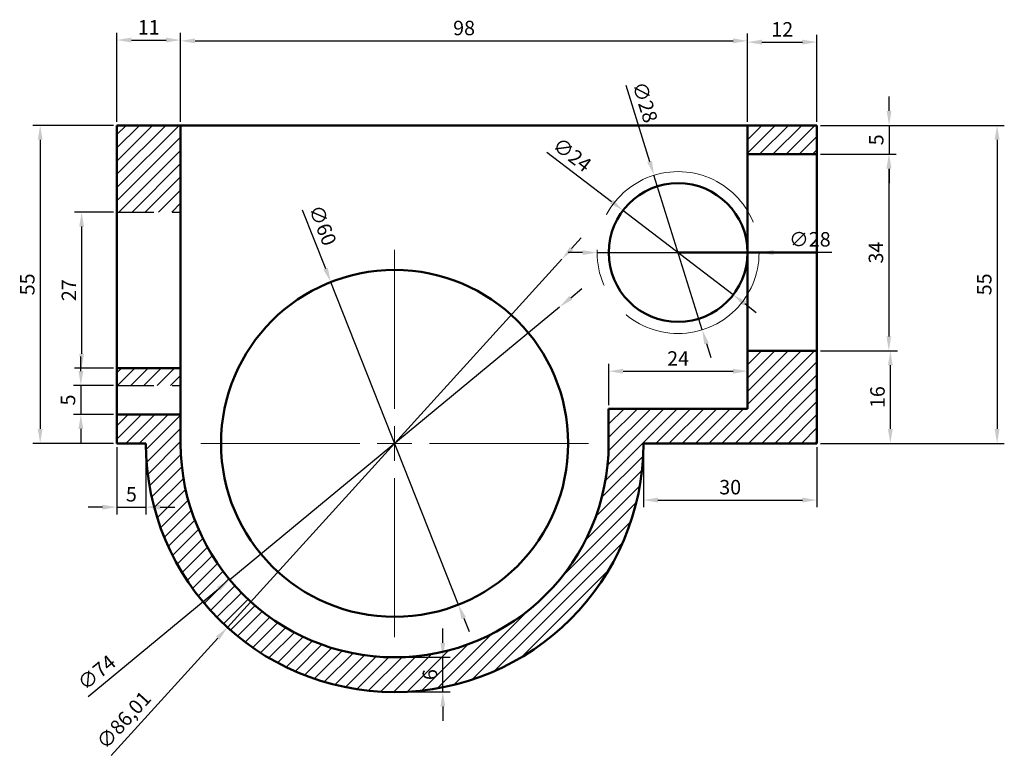
# Model space of a CAD drawing. Units: millimetres. Extents: x 1194 to 1920, y 1729 to 2086.
# Tile 5 of 5: x 1750 to 1920, y 1959 to 2086. Entities that reach past the tile are written whole.
import ezdxf

# ---------------------------------------------------------------- set-up
doc = ezdxf.new("R2010")
doc.units = ezdxf.units.MM
doc.linetypes.add('CENTER', pattern=[50.8, 31.75, -6.35, 6.35, -6.35])
doc.linetypes.add('HIDDEN', pattern=[9.525, 6.35, -3.175])
for name, color, linetype, lineweight in [('M-CNTR', 1, 'CENTER', 18), ('M-DIMS', 2, 'Continuous', 25), ('M-HATC', 8, 'Continuous', 18), ('M-HIDN', 4, 'HIDDEN', 25), ('M-OUTL', 7, 'Continuous', 50)]:
    doc.layers.add(name, color=color, linetype=linetype, lineweight=lineweight)
doc.styles.get("Standard").update_dxf_attribs({"font": 'arial.ttf'})
doc.dimstyles.new('ISO-25', dxfattribs={"dimtxt": 2.5, "dimasz": 2.5, "dimexe": 1.25, "dimexo": 0.625, "dimtad": 1, "dimtxsty": 'Standard', "dimcen": 2.5, "dimadec": 0, "dimazin": 0, "dimtfac": 1, "dimtmove": 0, "dimatfit": 3, "dimfxl": 1, "dimarcsym": 0})

# ---------------------------------------------------------------- blocks, each defined once
blk = doc.blocks.new('*U9')
at = {"layer": 'M-CNTR', "color": 0, "transparency": 16777216}
for p, q in [((0, 6), (0, 33.5)), ((-33.5, 0), (-6, 0)), ((6, 0), (33.5, 0)), ((0, -33.5), (0, -6))]:
    blk.add_line(p, q, dxfattribs=at)
at = {"layer": 'M-CNTR', "color": 0, "linetype": 'Continuous', "transparency": 16777216}
for p, q in [((0, -3), (0, 3)), ((-3, 0), (3, 0))]:
    blk.add_line(p, q, dxfattribs=at)
blk = doc.blocks.new('*D62')
at = {"layer": 'Defpoints', "color": 0, "transparency": 16777216}
for p in [(1777.47, 2082.79), (1766.46, 2068.03), (1777.47, 2068.03)]:
    blk.add_point(p, dxfattribs=at)
at = {"layer": 'M-DIMS', "color": 0, "lineweight": -2, "transparency": 16777216}
for p, q in [((1766.46, 2068.65), (1766.46, 2084.04)), ((1777.47, 2068.65), (1777.47, 2084.04)), ((1768.96, 2082.79), (1774.97, 2082.79))]:
    blk.add_line(p, q, dxfattribs=at)
at = {"layer": 'M-DIMS', "color": 0, "transparency": 16777216}
for points in [[(1768.96, 2083.21), (1768.96, 2082.37), (1766.46, 2082.79)], [(1774.97, 2083.21), (1774.97, 2082.37), (1777.47, 2082.79)]]:
    blk.add_solid(points, dxfattribs=at)
at = {"layer": 'M-DIMS', "color": 0, "transparency": 16777216, "insert": (1771.96, 2084.67), "char_height": 2.5, "attachment_point": 5}
blk.add_mtext('11', dxfattribs=at)
blk = doc.blocks.new('*D63')
at = {"layer": 'Defpoints', "color": 0, "transparency": 16777216}
for p in [(1875.47, 2082.65), (1777.47, 2068.03), (1875.47, 2068.03)]:
    blk.add_point(p, dxfattribs=at)
at = {"layer": 'M-DIMS', "color": 0, "lineweight": -2, "transparency": 16777216}
for p, q in [((1777.47, 2068.65), (1777.47, 2083.9)), ((1875.47, 2068.65), (1875.47, 2083.9)), ((1779.97, 2082.65), (1872.97, 2082.65))]:
    blk.add_line(p, q, dxfattribs=at)
at = {"layer": 'M-DIMS', "color": 0, "transparency": 16777216}
for points in [[(1779.97, 2083.07), (1779.97, 2082.23), (1777.47, 2082.65)], [(1872.97, 2083.07), (1872.97, 2082.23), (1875.47, 2082.65)]]:
    blk.add_solid(points, dxfattribs=at)
at = {"layer": 'M-DIMS', "color": 0, "transparency": 16777216, "insert": (1826.47, 2084.55), "char_height": 2.5, "attachment_point": 5}
blk.add_mtext('98', dxfattribs=at)
blk = doc.blocks.new('*D64')
at = {"layer": 'Defpoints', "color": 0, "transparency": 16777216}
for p in [(1887.47, 2082.43), (1875.47, 2068.03), (1887.47, 2068.03)]:
    blk.add_point(p, dxfattribs=at)
at = {"layer": 'M-DIMS', "color": 0, "lineweight": -2, "transparency": 16777216}
for p, q in [((1875.47, 2068.65), (1875.47, 2083.68)), ((1887.47, 2068.65), (1887.47, 2083.68)), ((1877.97, 2082.43), (1884.97, 2082.43))]:
    blk.add_line(p, q, dxfattribs=at)
at = {"layer": 'M-DIMS', "color": 0, "transparency": 16777216}
for points in [[(1877.97, 2082.85), (1877.97, 2082.01), (1875.47, 2082.43)], [(1884.97, 2082.85), (1884.97, 2082.01), (1887.47, 2082.43)]]:
    blk.add_solid(points, dxfattribs=at)
at = {"layer": 'M-DIMS', "color": 0, "transparency": 16777216, "insert": (1881.47, 2084.31), "char_height": 2.5, "attachment_point": 5}
blk.add_mtext('12', dxfattribs=at)
blk = doc.blocks.new('*D65')
at = {"layer": 'Defpoints', "color": 0, "transparency": 16777216}
for p in [(1887.47, 2068.03), (1887.47, 2013.03), (1918.61, 2013.03)]:
    blk.add_point(p, dxfattribs=at)
at = {"layer": 'M-DIMS', "color": 0, "lineweight": -2, "transparency": 16777216}
for p, q in [((1888.09, 2068.03), (1919.86, 2068.03)), ((1918.61, 2065.53), (1918.61, 2015.53)), ((1888.09, 2013.03), (1919.86, 2013.03))]:
    blk.add_line(p, q, dxfattribs=at)
at = {"layer": 'M-DIMS', "color": 0, "transparency": 16777216}
for points in [[(1918.19, 2065.53), (1919.03, 2065.53), (1918.61, 2068.03)], [(1918.19, 2015.53), (1919.03, 2015.53), (1918.61, 2013.03)]]:
    blk.add_solid(points, dxfattribs=at)
at = {"layer": 'M-DIMS', "color": 0, "transparency": 16777216, "insert": (1916.71, 2040.53), "char_height": 2.5, "attachment_point": 5, "rotation": 90}
blk.add_mtext('55', dxfattribs=at)
blk = doc.blocks.new('*D66')
at = {"layer": 'Defpoints', "color": 0, "transparency": 16777216}
for p in [(1887.47, 2068.03), (1887.47, 2063.03), (1899.94, 2063.03)]:
    blk.add_point(p, dxfattribs=at)
at = {"layer": 'M-DIMS', "color": 0, "lineweight": -2, "transparency": 16777216}
for p, q in [((1899.94, 2070.53), (1899.94, 2073.03)), ((1888.09, 2068.03), (1901.19, 2068.03)), ((1899.94, 2068.03), (1899.94, 2063.03)), ((1888.09, 2063.03), (1901.19, 2063.03)), ((1899.94, 2060.53), (1899.94, 2058.03))]:
    blk.add_line(p, q, dxfattribs=at)
at = {"layer": 'M-DIMS', "color": 0, "transparency": 16777216}
for points in [[(1899.52, 2070.53), (1900.36, 2070.53), (1899.94, 2068.03)], [(1899.52, 2060.53), (1900.36, 2060.53), (1899.94, 2063.03)]]:
    blk.add_solid(points, dxfattribs=at)
at = {"layer": 'M-DIMS', "color": 0, "transparency": 16777216, "insert": (1898.04, 2065.53), "char_height": 2.5, "attachment_point": 5, "rotation": 90}
blk.add_mtext('5', dxfattribs=at)
blk = doc.blocks.new('*D67')
at = {"layer": 'Defpoints', "color": 0, "transparency": 16777216}
for p in [(1887.47, 2029.03), (1900.16, 2029.03), (1887.47, 2013.03)]:
    blk.add_point(p, dxfattribs=at)
at = {"layer": 'M-DIMS', "color": 0, "lineweight": -2, "transparency": 16777216}
for p, q in [((1888.09, 2029.03), (1901.41, 2029.03)), ((1900.16, 2015.53), (1900.16, 2026.53)), ((1888.09, 2013.03), (1901.41, 2013.03))]:
    blk.add_line(p, q, dxfattribs=at)
at = {"layer": 'M-DIMS', "color": 0, "transparency": 16777216}
for points in [[(1899.74, 2026.53), (1900.57, 2026.53), (1900.16, 2029.03)], [(1899.74, 2015.53), (1900.57, 2015.53), (1900.16, 2013.03)]]:
    blk.add_solid(points, dxfattribs=at)
at = {"layer": 'M-DIMS', "color": 0, "transparency": 16777216, "insert": (1898.26, 2021.03), "char_height": 2.5, "attachment_point": 5, "rotation": 90}
blk.add_mtext('16', dxfattribs=at)
blk = doc.blocks.new('*D68')
at = {"layer": 'Defpoints', "color": 0, "transparency": 16777216}
for p in [(1766.46, 2013.03), (1771.46, 2013.03), (1771.46, 2002)]:
    blk.add_point(p, dxfattribs=at)
at = {"layer": 'M-DIMS', "color": 0, "lineweight": -2, "transparency": 16777216}
for p, q in [((1766.46, 2012.4), (1766.46, 2000.75)), ((1771.46, 2012.4), (1771.46, 2000.75)), ((1763.96, 2002), (1761.46, 2002)), ((1766.46, 2002), (1771.46, 2002)), ((1773.96, 2002), (1776.46, 2002))]:
    blk.add_line(p, q, dxfattribs=at)
at = {"layer": 'M-DIMS', "color": 0, "transparency": 16777216}
for points in [[(1763.96, 2002.42), (1763.96, 2001.58), (1766.46, 2002)], [(1773.96, 2002.42), (1773.96, 2001.58), (1771.46, 2002)]]:
    blk.add_solid(points, dxfattribs=at)
at = {"layer": 'M-DIMS', "color": 0, "transparency": 16777216, "insert": (1768.96, 2003.9), "char_height": 2.5, "attachment_point": 5}
blk.add_mtext('5', dxfattribs=at)
blk = doc.blocks.new('*D69')
at = {"layer": 'Defpoints', "color": 0, "transparency": 16777216}
for p in [(1766.46, 2068.03), (1753.19, 2013.03), (1766.46, 2013.03)]:
    blk.add_point(p, dxfattribs=at)
at = {"layer": 'M-DIMS', "color": 0, "lineweight": -2, "transparency": 16777216}
for p, q in [((1765.84, 2068.03), (1751.94, 2068.03)), ((1753.19, 2065.53), (1753.19, 2015.53)), ((1765.84, 2013.03), (1751.94, 2013.03))]:
    blk.add_line(p, q, dxfattribs=at)
at = {"layer": 'M-DIMS', "color": 0, "transparency": 16777216}
for points in [[(1752.77, 2065.53), (1753.61, 2065.53), (1753.19, 2068.03)], [(1752.77, 2015.53), (1753.61, 2015.53), (1753.19, 2013.03)]]:
    blk.add_solid(points, dxfattribs=at)
at = {"layer": 'M-DIMS', "color": 0, "transparency": 16777216, "insert": (1751.29, 2040.53), "char_height": 2.5, "attachment_point": 5, "rotation": 90}
blk.add_mtext('55', dxfattribs=at)
blk = doc.blocks.new('*D70')
at = {"layer": 'Defpoints', "color": 0, "transparency": 16777216}
for p in [(1766.46, 2053.03), (1760.36, 2026.03), (1766.46, 2026.03)]:
    blk.add_point(p, dxfattribs=at)
at = {"layer": 'M-DIMS', "color": 0, "lineweight": -2, "transparency": 16777216}
for p, q in [((1765.84, 2053.03), (1759.11, 2053.03)), ((1760.36, 2050.53), (1760.36, 2028.53)), ((1765.84, 2026.03), (1759.11, 2026.03))]:
    blk.add_line(p, q, dxfattribs=at)
at = {"layer": 'M-DIMS', "color": 0, "transparency": 16777216}
for points in [[(1759.94, 2050.53), (1760.78, 2050.53), (1760.36, 2053.03)], [(1759.94, 2028.53), (1760.78, 2028.53), (1760.36, 2026.03)]]:
    blk.add_solid(points, dxfattribs=at)
at = {"layer": 'M-DIMS', "color": 0, "transparency": 16777216, "insert": (1758.48, 2039.53), "char_height": 2.5, "attachment_point": 5, "rotation": 90}
blk.add_mtext('27', dxfattribs=at)
blk = doc.blocks.new('*D71')
at = {"layer": 'Defpoints', "color": 0, "transparency": 16777216}
for p in [(1766.46, 2023.03), (1760.22, 2018.03), (1766.46, 2018.03)]:
    blk.add_point(p, dxfattribs=at)
at = {"layer": 'M-DIMS', "color": 0, "lineweight": -2, "transparency": 16777216}
for p, q in [((1760.22, 2025.53), (1760.22, 2028.03)), ((1765.84, 2023.03), (1758.97, 2023.03)), ((1760.22, 2023.03), (1760.22, 2018.03)), ((1765.84, 2018.03), (1758.97, 2018.03)), ((1760.22, 2015.53), (1760.22, 2013.03))]:
    blk.add_line(p, q, dxfattribs=at)
at = {"layer": 'M-DIMS', "color": 0, "transparency": 16777216}
for points in [[(1759.81, 2025.53), (1760.64, 2025.53), (1760.22, 2023.03)], [(1759.81, 2015.53), (1760.64, 2015.53), (1760.22, 2018.03)]]:
    blk.add_solid(points, dxfattribs=at)
at = {"layer": 'M-DIMS', "color": 0, "transparency": 16777216, "insert": (1758.33, 2020.53), "char_height": 2.5, "attachment_point": 5, "rotation": 90}
blk.add_mtext('5', dxfattribs=at)
blk = doc.blocks.new('*D72')
at = {"layer": 'Defpoints', "color": 0, "transparency": 16777216}
for p in [(1875.47, 2025.51), (1851.47, 2019.03), (1875.47, 2019.03)]:
    blk.add_point(p, dxfattribs=at)
at = {"layer": 'M-DIMS', "color": 0, "lineweight": -2, "transparency": 16777216}
for p, q in [((1851.47, 2019.65), (1851.47, 2026.76)), ((1853.97, 2025.51), (1872.97, 2025.51)), ((1875.47, 2019.65), (1875.47, 2026.76))]:
    blk.add_line(p, q, dxfattribs=at)
at = {"layer": 'M-DIMS', "color": 0, "transparency": 16777216}
for points in [[(1853.97, 2025.93), (1853.97, 2025.09), (1851.47, 2025.51)], [(1872.97, 2025.93), (1872.97, 2025.09), (1875.47, 2025.51)]]:
    blk.add_solid(points, dxfattribs=at)
at = {"layer": 'M-DIMS', "color": 0, "transparency": 16777216, "insert": (1863.47, 2027.39), "char_height": 2.5, "attachment_point": 5}
blk.add_mtext('24', dxfattribs=at)
blk = doc.blocks.new('*D73')
at = {"layer": 'Defpoints', "color": 0, "transparency": 16777216}
for p in [(1857.47, 2013.03), (1887.47, 2013.03), (1887.47, 2003.22)]:
    blk.add_point(p, dxfattribs=at)
at = {"layer": 'M-DIMS', "color": 0, "lineweight": -2, "transparency": 16777216}
for p, q in [((1857.47, 2012.4), (1857.47, 2001.97)), ((1887.47, 2012.4), (1887.47, 2001.97)), ((1859.97, 2003.22), (1884.97, 2003.22))]:
    blk.add_line(p, q, dxfattribs=at)
at = {"layer": 'M-DIMS', "color": 0, "transparency": 16777216}
for points in [[(1859.97, 2003.64), (1859.97, 2002.81), (1857.47, 2003.22)], [(1884.97, 2003.64), (1884.97, 2002.81), (1887.47, 2003.22)]]:
    blk.add_solid(points, dxfattribs=at)
at = {"layer": 'M-DIMS', "color": 0, "transparency": 16777216, "insert": (1872.47, 2005.13), "char_height": 2.5, "attachment_point": 5}
blk.add_mtext('30', dxfattribs=at)
blk = doc.blocks.new('*D74')
at = {"layer": 'Defpoints', "color": 0, "transparency": 16777216}
for p in [(1887.47, 2063.03), (1887.47, 2029.03), (1899.9, 2029.03)]:
    blk.add_point(p, dxfattribs=at)
at = {"layer": 'M-DIMS', "color": 0, "lineweight": -2, "transparency": 16777216}
for p, q in [((1888.09, 2063.03), (1901.15, 2063.03)), ((1899.9, 2060.53), (1899.9, 2031.53)), ((1888.09, 2029.03), (1901.15, 2029.03))]:
    blk.add_line(p, q, dxfattribs=at)
at = {"layer": 'M-DIMS', "color": 0, "transparency": 16777216}
for points in [[(1899.48, 2060.53), (1900.31, 2060.53), (1899.9, 2063.03)], [(1899.48, 2031.53), (1900.31, 2031.53), (1899.9, 2029.03)]]:
    blk.add_solid(points, dxfattribs=at)
at = {"layer": 'M-DIMS', "color": 0, "transparency": 16777216, "insert": (1897.99, 2046.03), "char_height": 2.5, "attachment_point": 5, "rotation": 90}
blk.add_mtext('34', dxfattribs=at)
blk = doc.blocks.new('*D75')
at = {"layer": 'Defpoints', "color": 0, "transparency": 16777216}
for p in [(1853.94, 2053.33), (1872.99, 2038.73)]:
    blk.add_point(p, dxfattribs=at)
at = {"layer": 'M-DIMS', "color": 0, "lineweight": -2, "transparency": 16777216}
for p, q in [((1840.77, 2063.42), (1851.96, 2054.85)), ((1872.99, 2038.73), (1853.94, 2053.33)), ((1874.98, 2037.21), (1876.96, 2035.69))]:
    blk.add_line(p, q, dxfattribs=at)
at = {"layer": 'M-DIMS', "color": 0, "transparency": 16777216}
for points in [[(1852.21, 2055.18), (1851.71, 2054.52), (1853.94, 2053.33)], [(1875.23, 2037.54), (1874.72, 2036.88), (1872.99, 2038.73)]]:
    blk.add_solid(points, dxfattribs=at)
at = {"layer": 'M-DIMS', "color": 0, "transparency": 16777216, "insert": (1844.96, 2062.7), "char_height": 2.5, "attachment_point": 5, "rotation": 322.5372}
blk.add_mtext('∅24', dxfattribs=at)
blk = doc.blocks.new('*D76')
at = {"layer": 'Defpoints', "color": 0, "transparency": 16777216}
for p in [(1859.3, 2059.39), (1867.64, 2032.67)]:
    blk.add_point(p, dxfattribs=at)
at = {"layer": 'M-DIMS', "color": 0, "lineweight": -2, "transparency": 16777216}
for p, q in [((1854.43, 2074.97), (1858.55, 2061.78)), ((1867.64, 2032.67), (1859.3, 2059.39)), ((1868.39, 2030.28), (1869.13, 2027.89))]:
    blk.add_line(p, q, dxfattribs=at)
at = {"layer": 'M-DIMS', "color": 0, "transparency": 16777216}
for points in [[(1858.95, 2061.9), (1858.15, 2061.66), (1859.3, 2059.39)], [(1868.78, 2030.4), (1867.99, 2030.16), (1867.64, 2032.67)]]:
    blk.add_solid(points, dxfattribs=at)
at = {"layer": 'M-DIMS', "color": 0, "transparency": 16777216, "insert": (1857.44, 2071.95), "char_height": 2.5, "attachment_point": 5, "rotation": 287.3417}
blk.add_mtext('∅28', dxfattribs=at)
blk = doc.blocks.new('*D77')
at = {"layer": 'Defpoints', "color": 0, "transparency": 16777216}
for p in [(1803.44, 2040.93), (1825.49, 1985.13)]:
    blk.add_point(p, dxfattribs=at)
at = {"layer": 'M-DIMS', "color": 0, "lineweight": -2, "transparency": 16777216}
for p, q in [((1798.51, 2053.42), (1802.52, 2043.26)), ((1825.49, 1985.13), (1803.44, 2040.93)), ((1826.41, 1982.8), (1827.33, 1980.48))]:
    blk.add_line(p, q, dxfattribs=at)
at = {"layer": 'M-DIMS', "color": 0, "transparency": 16777216}
for points in [[(1802.91, 2043.41), (1802.13, 2043.1), (1803.44, 2040.93)], [(1826.8, 1982.96), (1826.02, 1982.65), (1825.49, 1985.13)]]:
    blk.add_solid(points, dxfattribs=at)
at = {"layer": 'M-DIMS', "color": 0, "transparency": 16777216, "insert": (1801.73, 2050.63), "char_height": 2.5, "attachment_point": 5, "rotation": 291.5599}
blk.add_mtext('∅60', dxfattribs=at)
blk = doc.blocks.new('*D78')
at = {"layer": 'Defpoints', "color": 0, "transparency": 16777216}
for p in [(1842.98, 2036.61), (1785.95, 1989.45)]:
    blk.add_point(p, dxfattribs=at)
at = {"layer": 'M-DIMS', "color": 0, "lineweight": -2, "transparency": 16777216}
for p, q in [((1844.9, 2038.2), (1846.83, 2039.8)), ((1842.98, 2036.61), (1785.95, 1989.45)), ((1761.51, 1969.23), (1784.03, 1987.85))]:
    blk.add_line(p, q, dxfattribs=at)
at = {"layer": 'M-DIMS', "color": 0, "transparency": 16777216}
for points in [[(1844.64, 2038.52), (1845.17, 2037.88), (1842.98, 2036.61)], [(1783.76, 1988.18), (1784.29, 1987.53), (1785.95, 1989.45)]]:
    blk.add_solid(points, dxfattribs=at)
at = {"layer": 'M-DIMS', "color": 0, "transparency": 16777216, "insert": (1763.16, 1973.15), "char_height": 2.5, "attachment_point": 5, "rotation": 39.5929}
blk.add_mtext('∅74', dxfattribs=at)
blk = doc.blocks.new('*D79')
at = {"layer": 'Defpoints', "color": 0, "transparency": 16777216}
for p in [(1843.37, 2044.87), (1785.56, 1981.19)]:
    blk.add_point(p, dxfattribs=at)
at = {"layer": 'M-DIMS', "color": 0, "lineweight": -2, "transparency": 16777216}
for p, q in [((1845.05, 2046.72), (1846.74, 2048.57)), ((1843.37, 2044.87), (1785.56, 1981.19)), ((1765.47, 1959.07), (1783.88, 1979.34))]:
    blk.add_line(p, q, dxfattribs=at)
at = {"layer": 'M-DIMS', "color": 0, "transparency": 16777216}
for points in [[(1844.75, 2047), (1845.36, 2046.44), (1843.37, 2044.87)], [(1783.57, 1979.62), (1784.18, 1979.06), (1785.56, 1981.19)]]:
    blk.add_solid(points, dxfattribs=at)
at = {"layer": 'M-DIMS', "color": 0, "transparency": 16777216, "insert": (1767.88, 1964.95), "char_height": 2.5, "attachment_point": 5, "rotation": 47.7595}
blk.add_mtext('∅86,01', dxfattribs=at)
blk = doc.blocks.new('*D80')
at = {"layer": 'Defpoints', "color": 0, "transparency": 16777216}
for p in [(1814.47, 1976.03), (1822.79, 1976.03), (1814.47, 1970.03)]:
    blk.add_point(p, dxfattribs=at)
at = {"layer": 'M-DIMS', "color": 0, "lineweight": -2, "transparency": 16777216}
for p, q in [((1822.79, 1978.53), (1822.79, 1981.03)), ((1815.09, 1976.03), (1824.04, 1976.03)), ((1822.79, 1970.03), (1822.79, 1976.03)), ((1815.09, 1970.03), (1824.04, 1970.03)), ((1822.79, 1967.53), (1822.79, 1965.03))]:
    blk.add_line(p, q, dxfattribs=at)
at = {"layer": 'M-DIMS', "color": 0, "transparency": 16777216}
for points in [[(1822.38, 1978.53), (1823.21, 1978.53), (1822.79, 1976.03)], [(1822.38, 1967.53), (1823.21, 1967.53), (1822.79, 1970.03)]]:
    blk.add_solid(points, dxfattribs=at)
at = {"layer": 'M-DIMS', "color": 0, "transparency": 16777216, "insert": (1820.89, 1973.03), "char_height": 2.5, "attachment_point": 5, "rotation": 90}
blk.add_mtext('6', dxfattribs=at)
blk = doc.blocks.new('*D149')
at = {"layer": 'Defpoints', "color": 0, "transparency": 16777216}
for p in [(1849.47, 2046.03), (1877.47, 2046.03)]:
    blk.add_point(p, dxfattribs=at)
at = {"layer": 'M-DIMS', "color": 0, "lineweight": -2, "transparency": 16777216}
for p, q in [((1846.97, 2046.03), (1844.47, 2046.03)), ((1849.47, 2046.03), (1877.47, 2046.03)), ((1890.02, 2046.03), (1879.97, 2046.03))]:
    blk.add_line(p, q, dxfattribs=at)
at = {"layer": 'M-DIMS', "color": 0, "transparency": 16777216}
for points in [[(1846.97, 2046.45), (1846.97, 2045.61), (1849.47, 2046.03)], [(1879.97, 2046.45), (1879.97, 2045.61), (1877.47, 2046.03)]]:
    blk.add_solid(points, dxfattribs=at)
at = {"layer": 'M-DIMS', "color": 0, "transparency": 16777216, "insert": (1886.25, 2048), "char_height": 2.5, "attachment_point": 5, "rotation": 359.9988}
blk.add_mtext('∅28', dxfattribs=at)

msp = doc.modelspace()

# ---------------------------------------------------------------- hatches: boundary and pattern name
at = {"layer": 'M-HATC'}
h = msp.add_hatch(dxfattribs=at)
h.set_pattern_fill('ANSI31', color=256, scale=0.51)
h.paths.add_polyline_path([(1771.462, 2013.0293), (1766.462, 2013.0293), (1766.462, 2018.0293), (1777.4653, 2018.0293), (1777.4653, 2013.0293, 1), (1851.4653, 2013.0293), (1851.4653, 2019.0293), (1875.4685, 2019.0293), (1875.4685, 2029.0293), (1887.4685, 2029.0293), (1887.4685, 2013.0293), (1857.4685, 2013.0293, -1)])
h.paths.add_polyline_path([(1887.4685, 2068.0293), (1875.4685, 2068.0293), (1875.4685, 2063.0293), (1887.4685, 2063.0293), (1887.4685, 2066.0293)])
h = msp.add_hatch(dxfattribs=at)
h.set_pattern_fill('ANSI31', color=256, scale=0.51)
h.paths.add_polyline_path([(1777.4653, 2068.0293), (1776.462, 2068.0293), (1766.462, 2068.0293), (1766.462, 2053.0293), (1777.4653, 2053.0293)])
h.paths.add_polyline_path([(1777.4653, 2026.0293), (1766.462, 2026.0293), (1766.462, 2023.0293), (1777.4653, 2023.0293)])

# ---------------------------------------------------------------- linework, layer by layer
at = {"layer": 'M-CNTR'}
msp.add_circle((1863.4685, 2046.0293), 14, dxfattribs=at)
at = {"layer": 'M-HIDN'}
for p, q in [((1766.462, 2068.0293), (1766.462, 2053.0293)), ((1766.462, 2053.0293), (1777.4653, 2053.0293)), ((1766.462, 2018.0293), (1766.462, 2023.0293)), ((1766.462, 2023.0293), (1777.4653, 2023.0293))]:
    msp.add_line(p, q, dxfattribs=at)
at = {"layer": 'M-OUTL'}
for p, q in [((1766.462, 2018.0293), (1766.462, 2068.0293)), ((1766.462, 2068.0293), (1776.462, 2068.0293)), ((1776.462, 2068.0293), (1777.4653, 2068.0293)), ((1777.4653, 2018.0293), (1777.4653, 2068.0293)), ((1777.4653, 2068.0293), (1887.4685, 2068.0293)), ((1887.4685, 2068.0293), (1875.4685, 2068.0293)), ((1875.4685, 2068.0293), (1875.4685, 2019.0293)), ((1875.4685, 2068.0293), (1875.4685, 2063.0293)), ((1887.4685, 2066.0293), (1887.4685, 2068.0293)), ((1887.4685, 2013.0293), (1887.4685, 2066.0293)), ((1875.4685, 2063.0293), (1887.4685, 2063.0293)), ((1887.4685, 2063.0293), (1887.4685, 2046.0293)), ((1875.4685, 2046.0293), (1863.4685, 2046.0293)), ((1887.4685, 2046.0293), (1875.4685, 2046.0293)), ((1875.4685, 2019.0293), (1875.4685, 2029.0293)), ((1875.4685, 2029.0293), (1887.4685, 2029.0293)), ((1777.4653, 2026.0293), (1766.462, 2026.0293)), ((1851.4653, 2013.0293), (1851.4653, 2019.0293)), ((1851.4653, 2019.0293), (1875.4685, 2019.0293)), ((1766.462, 2013.0293), (1766.462, 2018.0293)), ((1766.462, 2018.0293), (1777.4653, 2018.0293)), ((1777.4653, 2013.0293), (1777.4653, 2018.0293)), ((1771.462, 2013.0293), (1766.462, 2013.0293)), ((1857.4685, 2013.0293), (1887.4685, 2013.0293))]:
    msp.add_line(p, q, dxfattribs=at)
for centre, radius in [((1863.4685, 2046.0293), 12), ((1814.4653, 2013.0293), 30)]:
    msp.add_circle(centre, radius, dxfattribs=at)
for radius in [43.0033, 37]:
    msp.add_arc((1814.4653, 2013.0293), radius, 180, 0, dxfattribs=at)

# ---------------------------------------------------------------- block references
at = {"layer": 'M-CNTR'}
msp.add_blockref('*U9', (1814.4653, 2013.0293), dxfattribs=at)

# ---------------------------------------------------------------- dimensions: what is measured, and where the dimension line sits
at = {"layer": 'M-DIMS'}
for base, p1, p2, picture, middle in [((1777.4653, 2082.7908), (1766.462, 2068.0293), (1777.4653, 2068.0293), '*D62', (1771.9636, 2084.6709)), ((1875.4685, 2082.6486), (1777.4653, 2068.0293), (1875.4685, 2068.0293), '*D63', (1826.4669, 2084.5501)), ((1887.4685, 2082.4299), (1875.4685, 2068.0293), (1887.4685, 2068.0293), '*D64', (1881.4685, 2084.3101)), ((1875.4685, 2025.5109), (1851.4653, 2019.0293), (1875.4685, 2019.0293), '*D72', (1863.4669, 2027.391)), ((1771.462, 2002.0013), (1766.462, 2013.0293), (1771.462, 2013.0293), '*D68', (1768.962, 2003.8977)), ((1887.4685, 2003.2244), (1857.4685, 2013.0293), (1887.4685, 2013.0293), '*D73', (1872.4685, 2005.1267))]:
    dim = msp.add_linear_dim(base=base, p1=p1, p2=p2, dimstyle='ISO-25', override={"dimclrd": 0, "dimclre": 0, "dimclrt": 0}, dxfattribs=at)
    dim.commit()
    dim.dimension.update_dxf_attribs({"geometry": picture, "text_midpoint": middle})
for p1, p2, override, picture, middle in [((1867.6415, 2032.6657), (1859.2956, 2059.3929), {"dimclrd": 0, "dimclre": 0, "dimclrt": 0}, '*D76', (1855.5564, 2071.3673)), ((1872.9935, 2038.7303), (1853.9436, 2053.3282), {"dimclrd": 0, "dimclre": 0, "dimclrt": 0}, '*D75', (1843.7613, 2061.1308)), ((1825.4895, 1985.1283), (1803.441, 2040.9303), {"dimclrd": 0, "dimclre": 0, "dimclrt": 0}, '*D77', (1799.8937, 2049.9081)), ((1849.4685, 2046.0296), (1877.4685, 2046.029), {"dimdec": 0, "dimlfac": 1, "dimrnd": 0, "dimzin": 0, "dimdsep": 46, "dimlunit": 2}, '*D149', (1886.2467, 2046.0288)), ((1843.374, 2044.8659), (1785.5565, 1981.1927), {"dimclrd": 0, "dimclre": 0, "dimclrt": 0}, '*D79', (1769.4803, 1963.4882)), ((1842.9772, 2036.6104), (1785.9534, 1989.4481), {"dimclrd": 0, "dimclre": 0, "dimclrt": 0}, '*D78', (1764.413, 1971.6329))]:
    dim = msp.add_diameter_dim_2p(p1=p1, p2=p2, dimstyle='ISO-25', override=override, dxfattribs=at)
    dim.commit()
    dim.dimension.update_dxf_attribs({"geometry": picture, "text_midpoint": middle, "dimtype": 163})
for base, p1, p2, picture, middle in [((1899.9407, 2063.0293), (1887.4685, 2068.0293), (1887.4685, 2063.0293), '*D66', (1898.0444, 2065.5293)), ((1753.1884, 2013.0293), (1766.462, 2068.0293), (1766.462, 2013.0293), '*D69', (1751.2921, 2040.5293)), ((1918.6084, 2013.0293), (1887.4685, 2068.0293), (1887.4685, 2013.0293), '*D65', (1916.7121, 2040.5293)), ((1899.8951, 2029.0293), (1887.4685, 2063.0293), (1887.4685, 2029.0293), '*D74', (1897.9928, 2046.0293)), ((1760.3593, 2026.0293), (1766.462, 2053.0293), (1766.462, 2026.0293), '*D70', (1758.4792, 2039.5293)), ((1900.1578, 2029.0293), (1887.4685, 2013.0293), (1887.4685, 2029.0293), '*D67', (1898.2563, 2021.0293)), ((1760.2227, 2018.0293), (1766.462, 2023.0293), (1766.462, 2018.0293), '*D71', (1758.3264, 2020.5293))]:
    dim = msp.add_linear_dim(base=base, p1=p1, p2=p2, angle=90, dimstyle='ISO-25', override={"dimclrd": 0, "dimclre": 0, "dimclrt": 0}, dxfattribs=at)
    dim.commit()
    dim.dimension.update_dxf_attribs({"geometry": picture, "text_midpoint": middle})
dim = msp.add_aligned_dim(p1=(1814.4653, 1970.026), p2=(1814.4653, 1976.0293), distance=-8.3282, dimstyle='ISO-25', override={"dimclrd": 0, "dimclre": 0, "dimclrt": 0}, dxfattribs=at)
dim.commit()
dim.dimension.update_dxf_attribs({"geometry": '*D80', "text_midpoint": (1820.892, 1973.0277)})

doc.saveas('drawing.dxf')
